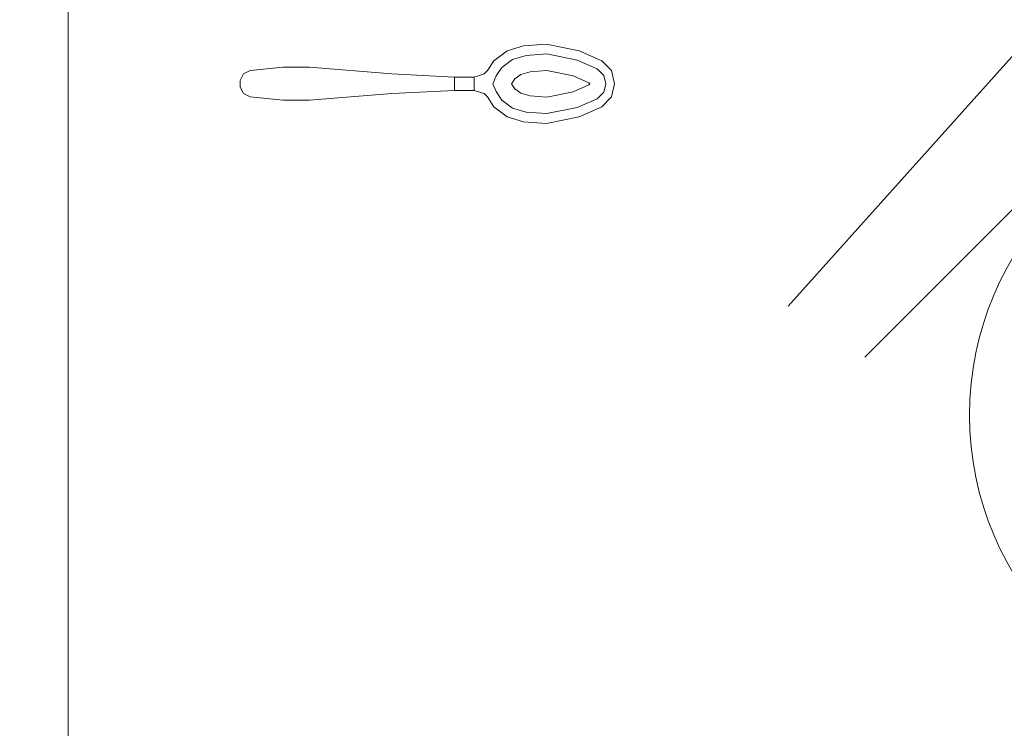
# Model space of a CAD drawing. Units: inches. Extents: x 375 to 1122, y 27 to 1069.
# Tile 26 of 155: x 705.14 to 720.91, y 285.2 to 296.54. Entities that reach past the tile are written whole.
import ezdxf

# ---------------------------------------------------------------- set-up
doc = ezdxf.new("R2010")
doc.units = ezdxf.units.IN
doc.layers.add('A-ANNO-DIMS', color=2, linetype='Continuous', lineweight=18)
doc.layers.add('Furniture', color=30, linetype='Continuous', lineweight=18)
doc.styles.get("Standard").update_dxf_attribs({"font": 'arial.ttf'})
doc.dimstyles.new('ISO-25', dxfattribs={"dimtxt": 12, "dimasz": 2.5, "dimexe": 1.5, "dimexo": 1.5, "dimtad": 1, "dimdec": 1, "dimlunit": 3, "dimtxsty": 'Standard', "dimblk": 'ARCHTICK', "dimcen": 2.5, "dimadec": 0, "dimazin": 0, "dimtfac": 1, "dimtdec": 1, "dimtmove": 0, "dimatfit": 3, "dimfxl": 1.5, "dimfxlon": 1, "dimarcsym": 0})

# ---------------------------------------------------------------- blocks, each defined once
blk = doc.blocks.new('A$C403C54AD')
for p, q in [((0.95931, 1.17062, -0.0006), (1.35847, 0.81256, -0.0006)), ((1.26636, 0.95578, -0.0006), (1.37894, 0.84325, -0.0006)), ((0.83575, 0.52421, -0.0006), (1.99923, 0.52421, -0.0006))]:
    blk.add_line(p, q)
blk.add_circle((1.40208, 1.00844, -0.0006), 0.12331)
for points, invisible_edges in [([(1.26354, 0.73605, -0.02421), (1.26029, 0.73789, -0.02157), (1.26425, 0.74173, -0.02048), (1.26622, 0.73867, -0.02365)], 5), ([(1.26354, 0.73605, -0.02289), (1.26029, 0.73789, -0.02025), (1.26425, 0.74173, -0.01916), (1.26622, 0.73867, -0.02233)], 5), ([(1.26425, 0.74173, -0.02048), (1.26622, 0.73867, -0.02365), (1.26953, 0.73948, -0.02346), (1.26953, 0.74304, -0.02029)], 5), ([(1.26425, 0.74173, -0.01916), (1.26622, 0.73867, -0.02233), (1.26953, 0.73948, -0.02215), (1.26953, 0.74304, -0.01897)], 5), ([(1.2748, 0.74173, -0.02048), (1.27283, 0.73867, -0.02365), (1.26953, 0.73948, -0.02346), (1.26953, 0.74304, -0.02029)], 5), ([(1.2748, 0.74173, -0.01916), (1.27283, 0.73867, -0.02233), (1.26953, 0.73948, -0.02215), (1.26953, 0.74304, -0.01897)], 5), ([(1.27551, 0.73605, -0.02421), (1.27876, 0.73789, -0.02157), (1.2748, 0.74173, -0.02048), (1.27283, 0.73867, -0.02365)], 5), ([(1.27551, 0.73605, -0.02289), (1.27876, 0.73789, -0.02025), (1.2748, 0.74173, -0.01916), (1.27283, 0.73867, -0.02233)], 5), ([(1.25633, 0.72882, -0.0234), (1.26003, 0.72802, -0.02592), (1.26354, 0.73605, -0.02421), (1.26029, 0.73789, -0.02157)], 5), ([(1.25633, 0.72882, -0.02208), (1.26003, 0.72802, -0.0246), (1.26354, 0.73605, -0.02289), (1.26029, 0.73789, -0.02025)], 5), ([(1.26909, 0.73267, -0.02578), (1.26622, 0.73867, -0.02233), (1.26354, 0.73605, -0.02289), (1.26909, 0.73267, -0.02578)], 5), ([(1.26909, 0.73267, -0.0271), (1.26622, 0.73867, -0.02365), (1.26354, 0.73605, -0.02421), (1.26909, 0.73267, -0.0271)], 5), ([(1.26953, 0.73948, -0.02215), (1.26953, 0.73309, -0.02564), (1.26909, 0.73267, -0.02578), (1.26622, 0.73867, -0.02233)], 5), ([(1.26953, 0.73948, -0.02346), (1.26953, 0.73309, -0.02696), (1.26909, 0.73267, -0.0271), (1.26622, 0.73867, -0.02365)], 5), ([(1.26953, 0.73948, -0.02215), (1.26953, 0.73309, -0.02564), (1.26996, 0.73267, -0.02578), (1.27283, 0.73867, -0.02233)], 5), ([(1.26953, 0.73948, -0.02346), (1.26953, 0.73309, -0.02696), (1.26996, 0.73267, -0.0271), (1.27283, 0.73867, -0.02365)], 5), ([(1.26996, 0.73267, -0.02578), (1.27283, 0.73867, -0.02233), (1.27551, 0.73605, -0.02289), (1.26996, 0.73267, -0.02578)], 5), ([(1.26996, 0.73267, -0.0271), (1.27283, 0.73867, -0.02365), (1.27551, 0.73605, -0.02421), (1.26996, 0.73267, -0.0271)], 5), ([(1.28272, 0.72882, -0.0234), (1.27902, 0.72802, -0.02592), (1.27551, 0.73605, -0.02421), (1.27876, 0.73789, -0.02157)], 5), ([(1.28272, 0.72882, -0.02208), (1.27902, 0.72802, -0.0246), (1.27551, 0.73605, -0.02289), (1.27876, 0.73789, -0.02025)], 5), ([(1.26354, 0.73605, -0.02421), (1.26909, 0.73267, -0.0271), (1.26635, 0.72644, -0.02873), (1.26003, 0.72802, -0.02592)], 5), ([(1.26354, 0.73605, -0.02289), (1.26909, 0.73267, -0.02578), (1.26635, 0.72644, -0.02741), (1.26003, 0.72802, -0.0246)], 5), ([(1.27551, 0.73605, -0.02421), (1.26996, 0.73267, -0.0271), (1.2727, 0.72644, -0.02873), (1.27902, 0.72802, -0.02592)], 5), ([(1.27551, 0.73605, -0.02289), (1.26996, 0.73267, -0.02578), (1.2727, 0.72644, -0.02741), (1.27902, 0.72802, -0.0246)], 5), ([(1.26909, 0.73267, -0.0271), (1.26996, 0.73267, -0.0271), (1.2727, 0.72644, -0.02873), (1.26635, 0.72644, -0.02873)], 5), ([(1.26909, 0.73267, -0.02578), (1.26996, 0.73267, -0.02578), (1.2727, 0.72644, -0.02741), (1.26635, 0.72644, -0.02741)], 5), ([(1.26953, 0.73309, -0.02564), (1.26996, 0.73267, -0.02578), (1.26909, 0.73267, -0.02578), (1.26953, 0.73309, -0.02564)], 2), ([(1.26953, 0.73309, -0.02696), (1.26996, 0.73267, -0.0271), (1.26909, 0.73267, -0.0271), (1.26953, 0.73309, -0.02696)], 2), ([(1.25757, 0.71589, -0.0279), (1.25369, 0.71579, -0.02544), (1.25633, 0.72882, -0.0234), (1.26003, 0.72802, -0.02592)], 5), ([(1.25757, 0.71589, -0.02658), (1.25369, 0.71579, -0.02412), (1.25633, 0.72882, -0.02208), (1.26003, 0.72802, -0.0246)], 5), ([(1.26635, 0.72644, -0.02741), (1.26003, 0.72802, -0.0246), (1.25757, 0.71589, -0.02658), (1.2642, 0.71583, -0.02912)], 5), ([(1.26635, 0.72644, -0.02873), (1.26003, 0.72802, -0.02592), (1.25757, 0.71589, -0.0279), (1.2642, 0.71583, -0.03044)], 5), ([(1.2727, 0.72644, -0.02741), (1.26635, 0.72644, -0.02741), (1.2642, 0.71583, -0.02912), (1.27485, 0.71583, -0.02912)], 5), ([(1.2727, 0.72644, -0.02873), (1.26635, 0.72644, -0.02873), (1.2642, 0.71583, -0.03044), (1.27485, 0.71583, -0.03044)], 5), ([(1.2727, 0.72644, -0.02741), (1.27902, 0.72802, -0.0246), (1.28148, 0.71589, -0.02658), (1.27485, 0.71583, -0.02912)], 5), ([(1.2727, 0.72644, -0.02873), (1.27902, 0.72802, -0.02592), (1.28148, 0.71589, -0.0279), (1.27485, 0.71583, -0.03044)], 5), ([(1.28148, 0.71589, -0.0279), (1.28536, 0.71579, -0.02544), (1.28272, 0.72882, -0.0234), (1.27902, 0.72802, -0.02592)], 5), ([(1.28148, 0.71589, -0.02658), (1.28536, 0.71579, -0.02412), (1.28272, 0.72882, -0.02208), (1.27902, 0.72802, -0.0246)], 5), ([(1.25435, 0.70658, -0.02499), (1.25817, 0.70765, -0.02747), (1.25757, 0.71589, -0.02658), (1.25369, 0.71579, -0.02412)], 5), ([(1.25435, 0.70658, -0.02631), (1.25817, 0.70765, -0.02879), (1.25757, 0.71589, -0.0279), (1.25369, 0.71579, -0.02544)], 5), ([(1.25757, 0.71589, -0.0279), (1.2642, 0.71583, -0.03044), (1.26468, 0.70922, -0.03139), (1.25817, 0.70765, -0.02879)], 5), ([(1.25757, 0.71589, -0.02658), (1.2642, 0.71583, -0.02912), (1.26468, 0.70922, -0.03007), (1.25817, 0.70765, -0.02747)], 5), ([(1.2642, 0.71583, -0.03044), (1.27485, 0.71583, -0.03044), (1.27437, 0.70922, -0.03139), (1.26468, 0.70922, -0.03139)], 5), ([(1.2642, 0.71583, -0.02912), (1.27485, 0.71583, -0.02912), (1.27437, 0.70922, -0.03007), (1.26468, 0.70922, -0.03007)], 5), ([(1.28148, 0.71589, -0.0279), (1.27485, 0.71583, -0.03044), (1.27437, 0.70922, -0.03139), (1.28088, 0.70765, -0.02879)], 5), ([(1.28148, 0.71589, -0.02658), (1.27485, 0.71583, -0.02912), (1.27437, 0.70922, -0.03007), (1.28088, 0.70765, -0.02747)], 5), ([(1.2847, 0.70658, -0.02499), (1.28088, 0.70765, -0.02747), (1.28148, 0.71589, -0.02658), (1.28536, 0.71579, -0.02412)], 5), ([(1.2847, 0.70658, -0.02631), (1.28088, 0.70765, -0.02879), (1.28148, 0.71589, -0.0279), (1.28536, 0.71579, -0.02544)], 5), ([(1.25983, 0.70213, -0.02798), (1.25633, 0.69998, -0.02539), (1.25435, 0.70658, -0.02499), (1.25817, 0.70765, -0.02747)], 5), ([(1.25983, 0.70213, -0.0293), (1.25633, 0.69998, -0.02671), (1.25435, 0.70658, -0.02631), (1.25817, 0.70765, -0.02879)], 5), ([(1.26468, 0.70922, -0.03007), (1.25817, 0.70765, -0.02747), (1.25983, 0.70213, -0.02798), (1.26579, 0.7055, -0.0303)], 5), ([(1.27437, 0.70922, -0.03139), (1.26468, 0.70922, -0.03139), (1.26579, 0.7055, -0.03162), (1.27326, 0.7055, -0.03162)], 5), ([(1.27437, 0.70922, -0.03007), (1.26468, 0.70922, -0.03007), (1.26579, 0.7055, -0.0303), (1.27326, 0.7055, -0.0303)], 5), ([(1.27437, 0.70922, -0.03139), (1.28088, 0.70765, -0.02879), (1.27922, 0.70213, -0.0293), (1.27326, 0.7055, -0.03162)], 5), ([(1.27437, 0.70922, -0.03007), (1.28088, 0.70765, -0.02747), (1.27922, 0.70213, -0.02798), (1.27326, 0.7055, -0.0303)], 5), ([(1.27922, 0.70213, -0.02798), (1.28272, 0.69998, -0.02539), (1.2847, 0.70658, -0.02499), (1.28088, 0.70765, -0.02747)], 5), ([(1.27922, 0.70213, -0.0293), (1.28272, 0.69998, -0.02671), (1.2847, 0.70658, -0.02631), (1.28088, 0.70765, -0.02879)], 5), ([(1.26029, 0.69472, -0.02719), (1.26298, 0.69791, -0.02947), (1.25983, 0.70213, -0.0293), (1.25633, 0.69998, -0.02671)], 5), ([(1.26029, 0.69472, -0.02588), (1.26298, 0.69791, -0.02815), (1.25983, 0.70213, -0.02798), (1.25633, 0.69998, -0.02539)], 5), ([(1.25983, 0.70213, -0.0293), (1.26579, 0.7055, -0.03162), (1.26756, 0.70313, -0.03172), (1.26298, 0.69791, -0.02947)], 5), ([(1.25983, 0.70213, -0.02798), (1.26579, 0.7055, -0.0303), (1.26756, 0.70313, -0.0304), (1.26298, 0.69791, -0.02815)], 5), ([(1.26756, 0.70313, -0.03172), (1.26298, 0.69791, -0.02947), (1.26639, 0.69562, -0.02948), (1.26953, 0.70178, -0.03152)], 5), ([(1.26756, 0.70313, -0.0304), (1.26298, 0.69791, -0.02815), (1.26639, 0.69562, -0.02816), (1.26953, 0.70178, -0.0302)], 5), ([(1.26579, 0.7055, -0.03162), (1.27326, 0.7055, -0.03162), (1.27149, 0.70313, -0.03172), (1.26756, 0.70313, -0.03172)], 5), ([(1.26579, 0.7055, -0.0303), (1.27326, 0.7055, -0.0303), (1.27149, 0.70313, -0.0304), (1.26756, 0.70313, -0.0304)], 5), ([(1.26639, 0.69562, -0.02948), (1.26953, 0.70178, -0.03152), (1.26953, 0.70178, -0.03152), (1.26953, 0.69426, -0.0293)], 5), ([(1.26639, 0.69562, -0.02816), (1.26953, 0.70178, -0.0302), (1.26953, 0.70178, -0.0302), (1.26953, 0.69426, -0.02798)], 5), ([(1.27149, 0.70313, -0.03172), (1.26756, 0.70313, -0.03172), (1.26953, 0.70178, -0.03152)], 1), ([(1.27149, 0.70313, -0.0304), (1.26756, 0.70313, -0.0304), (1.26953, 0.70178, -0.0302)], 1), ([(1.27149, 0.70313, -0.03172), (1.27607, 0.69791, -0.02947), (1.27266, 0.69562, -0.02948), (1.26953, 0.70178, -0.03152)], 5), ([(1.27149, 0.70313, -0.0304), (1.27607, 0.69791, -0.02815), (1.27266, 0.69562, -0.02816), (1.26953, 0.70178, -0.0302)], 5), ([(1.27266, 0.69562, -0.02948), (1.26953, 0.70178, -0.03152), (1.26953, 0.70178, -0.03152), (1.26953, 0.69426, -0.0293)], 5), ([(1.27266, 0.69562, -0.02816), (1.26953, 0.70178, -0.0302), (1.26953, 0.70178, -0.0302), (1.26953, 0.69426, -0.02798)], 5), ([(1.27922, 0.70213, -0.0293), (1.27326, 0.7055, -0.03162), (1.27149, 0.70313, -0.03172), (1.27607, 0.69791, -0.02947)], 5), ([(1.27922, 0.70213, -0.02798), (1.27326, 0.7055, -0.0303), (1.27149, 0.70313, -0.0304), (1.27607, 0.69791, -0.02815)], 5), ([(1.27876, 0.69472, -0.02719), (1.27607, 0.69791, -0.02947), (1.27922, 0.70213, -0.0293), (1.28272, 0.69998, -0.02671)], 5), ([(1.27876, 0.69472, -0.02588), (1.27607, 0.69791, -0.02815), (1.27922, 0.70213, -0.02798), (1.28272, 0.69998, -0.02539)], 5), ([(1.26639, 0.69562, -0.02816), (1.26425, 0.6921, -0.02625), (1.26029, 0.69472, -0.02588), (1.26298, 0.69791, -0.02815)], 5), ([(1.27266, 0.69562, -0.02948), (1.2748, 0.6921, -0.0284), (1.27876, 0.69472, -0.02719), (1.27607, 0.69791, -0.02947)], 5), ([(1.27266, 0.69562, -0.02816), (1.2748, 0.6921, -0.02625), (1.27876, 0.69472, -0.02588), (1.27607, 0.69791, -0.02815)], 5), ([(1.26425, 0.6921, -0.0284), (1.26953, 0.6921, -0.0284), (1.26953, 0.69426, -0.0293), (1.26639, 0.69562, -0.02948)], 11), ([(1.26425, 0.6921, -0.02625), (1.26953, 0.6921, -0.02625), (1.26953, 0.69426, -0.02798), (1.26639, 0.69562, -0.02816)], 11), ([(1.2748, 0.6921, -0.0284), (1.26953, 0.6921, -0.0284), (1.26953, 0.69426, -0.0293), (1.27266, 0.69562, -0.02948)], 11), ([(1.2748, 0.6921, -0.02625), (1.26953, 0.6921, -0.02625), (1.26953, 0.69426, -0.02798), (1.27266, 0.69562, -0.02816)], 11), ([(1.26557, 0.69077, -0.02551), (1.27348, 0.69077, -0.02551), (1.2748, 0.6921, -0.02625), (1.26425, 0.6921, -0.02625)], 5), ([(1.26557, 0.69077, -0.0276), (1.27348, 0.69077, -0.0276), (1.2748, 0.6921, -0.0284), (1.26425, 0.6921, -0.0284)], 5), ([(1.26557, 0.69077, -0.02551), (1.26557, 0.69077, -0.0276), (1.26425, 0.6921, -0.0284), (1.26425, 0.6921, -0.02625)], 1), ([(1.27216, 0.68681, -0.02366), (1.26689, 0.68681, -0.02366), (1.26557, 0.69077, -0.02551), (1.27348, 0.69077, -0.02551)], 4), ([(1.26689, 0.68681, -0.02588), (1.26689, 0.68681, -0.02366), (1.26557, 0.69077, -0.02551), (1.26557, 0.69077, -0.0276)], 5), ([(1.27216, 0.68681, -0.02588), (1.26689, 0.68681, -0.02588), (1.26557, 0.69077, -0.0276), (1.27348, 0.69077, -0.0276)], 4), ([(1.27216, 0.68681, -0.02366), (1.27216, 0.68681, -0.02588), (1.27348, 0.69077, -0.0276), (1.27348, 0.69077, -0.02551)], 5), ([(1.27348, 0.69077, -0.0276), (1.27348, 0.69077, -0.02551), (1.2748, 0.6921, -0.02625), (1.2748, 0.6921, -0.0284)], 1), ([(1.26689, 0.68681, -0.02588), (1.26689, 0.68681, -0.02366), (1.26689, 0.6789, -0.02303), (1.26689, 0.6789, -0.02525)], 5), ([(1.27216, 0.6789, -0.02525), (1.27216, 0.6789, -0.02303), (1.27216, 0.68681, -0.02366), (1.27216, 0.68681, -0.02588)], 5), ([(1.27348, 0.65383, -0.02553), (1.26557, 0.65383, -0.02553), (1.26689, 0.6789, -0.02303), (1.27216, 0.6789, -0.02303)], 1), ([(1.26689, 0.6789, -0.02303), (1.26689, 0.6789, -0.02525), (1.26557, 0.65383, -0.02816), (1.26557, 0.65383, -0.02553)], 5), ([(1.27348, 0.65383, -0.02816), (1.26557, 0.65383, -0.02816), (1.26689, 0.6789, -0.02525), (1.27216, 0.6789, -0.02525)], 1), ([(1.27348, 0.65383, -0.02553), (1.27348, 0.65383, -0.02816), (1.27216, 0.6789, -0.02525), (1.27216, 0.6789, -0.02303)], 5), ([(1.26293, 0.62085, -0.03154), (1.27612, 0.62085, -0.03154), (1.27348, 0.65383, -0.02816), (1.26557, 0.65383, -0.02816)], 5), ([(1.26557, 0.65383, -0.02816), (1.26557, 0.65383, -0.02553), (1.26293, 0.62085, -0.02757), (1.26293, 0.62085, -0.03154)], 1), ([(1.26293, 0.62085, -0.02757), (1.27612, 0.62085, -0.02757), (1.27348, 0.65383, -0.02553), (1.26557, 0.65383, -0.02553)], 5), ([(1.27612, 0.62085, -0.03154), (1.27612, 0.62085, -0.02757), (1.27348, 0.65383, -0.02553), (1.27348, 0.65383, -0.02816)], 4), ([(1.27612, 0.61029, -0.02785), (1.26293, 0.61029, -0.02785), (1.26293, 0.62085, -0.02757), (1.27612, 0.62085, -0.02757)], 5), ([(1.27612, 0.61029, -0.03182), (1.26293, 0.61029, -0.03182), (1.26293, 0.62085, -0.03154), (1.27612, 0.62085, -0.03154)], 5), ([(1.26425, 0.5971, -0.02782), (1.2748, 0.5971, -0.02782), (1.27612, 0.61029, -0.02785), (1.26293, 0.61029, -0.02785)], 5), ([(1.26425, 0.5971, -0.03179), (1.2748, 0.5971, -0.03179), (1.27612, 0.61029, -0.03182), (1.26293, 0.61029, -0.03182)], 5), ([(1.27348, 0.59446, -0.02761), (1.26557, 0.59446, -0.02761), (1.26425, 0.5971, -0.02782), (1.2748, 0.5971, -0.02782)], 5), ([(1.27348, 0.59446, -0.03158), (1.26557, 0.59446, -0.03158), (1.26425, 0.5971, -0.03179), (1.2748, 0.5971, -0.03179)], 5), ([(1.26821, 0.59314, -0.02775), (1.27084, 0.59314, -0.02775), (1.27348, 0.59446, -0.02761), (1.26557, 0.59446, -0.02761)], 4), ([(1.26821, 0.59314, -0.0313), (1.27084, 0.59314, -0.0313), (1.27348, 0.59446, -0.03158), (1.26557, 0.59446, -0.03158)], 4)]:
    blk.add_3dface(points, dxfattribs=dict(invisible_edges=invisible_edges))
for points in [[(1.26425, 0.74173, -0.01916), (1.26425, 0.74173, -0.02048), (1.26029, 0.73789, -0.02157), (1.26029, 0.73789, -0.02025)], [(1.26953, 0.74304, -0.02029), (1.26953, 0.74304, -0.01897), (1.26425, 0.74173, -0.01916), (1.26425, 0.74173, -0.02048)], [(1.2748, 0.74173, -0.01916), (1.2748, 0.74173, -0.02048), (1.26953, 0.74304, -0.02029), (1.26953, 0.74304, -0.01897)], [(1.27876, 0.73789, -0.02157), (1.27876, 0.73789, -0.02025), (1.2748, 0.74173, -0.01916), (1.2748, 0.74173, -0.02048)], [(1.26029, 0.73789, -0.02157), (1.26029, 0.73789, -0.02025), (1.25633, 0.72882, -0.02208), (1.25633, 0.72882, -0.0234)], [(1.28272, 0.72882, -0.02208), (1.28272, 0.72882, -0.0234), (1.27876, 0.73789, -0.02157), (1.27876, 0.73789, -0.02025)], [(1.25633, 0.72882, -0.02208), (1.25633, 0.72882, -0.0234), (1.25369, 0.71579, -0.02544), (1.25369, 0.71579, -0.02412)], [(1.28536, 0.71579, -0.02544), (1.28536, 0.71579, -0.02412), (1.28272, 0.72882, -0.02208), (1.28272, 0.72882, -0.0234)], [(1.25369, 0.71579, -0.02544), (1.25369, 0.71579, -0.02412), (1.25435, 0.70658, -0.02499), (1.25435, 0.70658, -0.02631)], [(1.2847, 0.70658, -0.02499), (1.2847, 0.70658, -0.02631), (1.28536, 0.71579, -0.02544), (1.28536, 0.71579, -0.02412)], [(1.25435, 0.70658, -0.02631), (1.25435, 0.70658, -0.02499), (1.25633, 0.69998, -0.02539), (1.25633, 0.69998, -0.02671)], [(1.28272, 0.69998, -0.02671), (1.28272, 0.69998, -0.02539), (1.2847, 0.70658, -0.02499), (1.2847, 0.70658, -0.02631)], [(1.25633, 0.69998, -0.02539), (1.25633, 0.69998, -0.02671), (1.26029, 0.69472, -0.02719), (1.26029, 0.69472, -0.02588)], [(1.27876, 0.69472, -0.02588), (1.27876, 0.69472, -0.02719), (1.28272, 0.69998, -0.02671), (1.28272, 0.69998, -0.02539)], [(1.26029, 0.69472, -0.02719), (1.26029, 0.69472, -0.02588), (1.26425, 0.6921, -0.02625), (1.26425, 0.6921, -0.0284)], [(1.2748, 0.6921, -0.0284), (1.2748, 0.6921, -0.02625), (1.27876, 0.69472, -0.02588), (1.27876, 0.69472, -0.02719)], [(1.26689, 0.6789, -0.02525), (1.27216, 0.6789, -0.02525), (1.27216, 0.68681, -0.02588), (1.26689, 0.68681, -0.02588)], [(1.26689, 0.6789, -0.02303), (1.27216, 0.6789, -0.02303), (1.27216, 0.68681, -0.02366), (1.26689, 0.68681, -0.02366)], [(1.26293, 0.62085, -0.02757), (1.26293, 0.62085, -0.03154), (1.26293, 0.61029, -0.03182), (1.26293, 0.61029, -0.02785)], [(1.27612, 0.61029, -0.02785), (1.27612, 0.61029, -0.03182), (1.27612, 0.62085, -0.03154), (1.27612, 0.62085, -0.02757)], [(1.26293, 0.61029, -0.03182), (1.26293, 0.61029, -0.02785), (1.26425, 0.5971, -0.02782), (1.26425, 0.5971, -0.03179)], [(1.2748, 0.5971, -0.03179), (1.2748, 0.5971, -0.02782), (1.27612, 0.61029, -0.02785), (1.27612, 0.61029, -0.03182)], [(1.26425, 0.5971, -0.02782), (1.26425, 0.5971, -0.03179), (1.26557, 0.59446, -0.03158), (1.26557, 0.59446, -0.02761)], [(1.27348, 0.59446, -0.02761), (1.27348, 0.59446, -0.03158), (1.2748, 0.5971, -0.03179), (1.2748, 0.5971, -0.02782)], [(1.26557, 0.59446, -0.03158), (1.26557, 0.59446, -0.02761), (1.26821, 0.59314, -0.02775), (1.26821, 0.59314, -0.0313)], [(1.26821, 0.59314, -0.02775), (1.26821, 0.59314, -0.0313), (1.27084, 0.59314, -0.0313), (1.27084, 0.59314, -0.02775)], [(1.27084, 0.59314, -0.0313), (1.27084, 0.59314, -0.02775), (1.27348, 0.59446, -0.02761), (1.27348, 0.59446, -0.03158)]]:
    blk.add_3dface(points)
blk = doc.blocks.new('_ArchTick')
at = {"color": 0, "linetype": 'ByBlock', "const_width": 0.15}
blk.add_lwpolyline([(-0.5, -0.5), (0.5, 0.5)], dxfattribs=at)
blk = doc.blocks.new('*D59')
at = {"layer": 'A-ANNO-DIMS', "color": 0, "lineweight": -2, "transparency": 16777216}
for p, q in [((668.717, 346.851), (665.717, 346.851)), ((667.217, 346.851), (667.217, 232.348)), ((668.717, 232.348), (665.717, 232.348)), ((667.217, 232.348), (667.217, 27.496))]:
    blk.add_line(p, q, dxfattribs=at)
at = {"layer": 'Defpoints', "color": 0, "transparency": 16777216}
for p in [(684.392, 346.851), (667.217, 232.348), (684.392, 232.348)]:
    blk.add_point(p, dxfattribs=at)
at = {"layer": 'A-ANNO-DIMS', "color": 0, "lineweight": -2, "transparency": 16777216, "xscale": 2.5, "yscale": 2.5, "zscale": 2.5}
for p, rotation in [((667.217, 346.851), 90), ((667.217, 232.348), 270)]:
    blk.add_blockref('_ArchTick', p, dxfattribs=dict(at, rotation=rotation))
at = {"layer": 'A-ANNO-DIMS', "color": 0, "transparency": 16777216, "insert": (660.387, 128.672), "char_height": 12, "attachment_point": 5, "rotation": 90}
blk.add_mtext('DINING SET 9\'-6 1/2" TYP.', dxfattribs=at)

msp = doc.modelspace()

# ---------------------------------------------------------------- block references
at = {"layer": 'Furniture', "xscale": 39.9918517141215, "yscale": 39.9918517141215, "zscale": 39.9918517141215, "rotation": 270}
msp.add_blockref('A$C403C54AD', (684.955, 346.287, 0.024), dxfattribs=at)

# ---------------------------------------------------------------- dimensions: what is measured, and where the dimension line sits
at = {"layer": 'A-ANNO-DIMS'}
dim = msp.add_linear_dim(base=(667.217, 232.348), p1=(684.392, 346.851), p2=(684.392, 232.348), angle=270, text='DINING SET <> TYP.', dimstyle='ISO-25', override={"dimdec": 1, "dimlfac": 1, "dimrnd": 0, "dimzin": 1, "dimdsep": 46, "dimlunit": 4, "dimfrac": 2}, dxfattribs=at)
dim.commit()
dim.dimension.update_dxf_attribs({"geometry": '*D59', "text_midpoint": (660.387, 128.672)})

doc.saveas('drawing.dxf')
